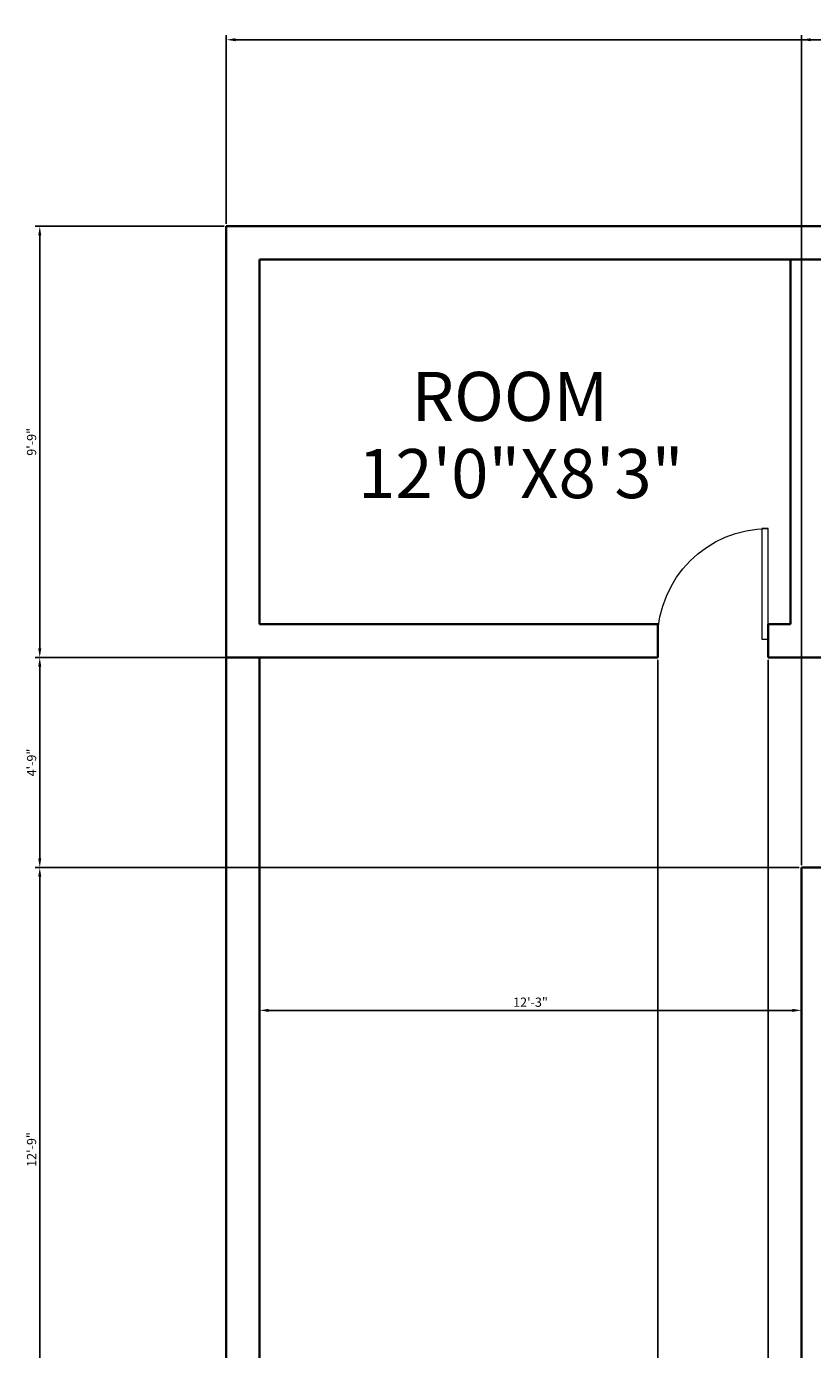
# Model space of a CAD drawing. Units: inches. Extents: x 3412 to 4225, y 13529 to 14581.
# Tile 4 of 7: x 3414 to 3627, y 14222 to 14581. Entities that reach past the tile are written whole.
import ezdxf

# ---------------------------------------------------------------- set-up
doc = ezdxf.new("R2010")
doc.units = ezdxf.units.IN
for name, color, linetype, lineweight in [('A-ANNO-DIMS', 2, 'Continuous', 13), ('A-AREA-IDEN', 7, 'Continuous', 18), ('A-DOOR', 4, 'Continuous', 18), ('A-WALL', 7, 'Continuous', 35), ('C-SITE-WALL', 7, 'Continuous', 35)]:
    doc.layers.add(name, color=color, linetype=linetype, lineweight=lineweight)
doc.styles.get("Standard").update_dxf_attribs({"font": 'arial.ttf'})
doc.dimstyles.new('ISO-25', dxfattribs={"dimtxt": 2.5, "dimasz": 2.5, "dimexe": 1.25, "dimexo": 0.625, "dimtad": 1, "dimdec": 0, "dimlunit": 3, "dimtxsty": 'Standard', "dimcen": 2.5, "dimadec": 0, "dimazin": 0, "dimtfac": 1, "dimtdec": 0, "dimtmove": 0, "dimatfit": 3, "dimfxl": 1, "dimarcsym": 0})

# ---------------------------------------------------------------- blocks, each defined once
blk = doc.blocks.new('*U3')
for p, q in [((0, 0), (0, -5)), ((30, 0), (30, -5))]:
    blk.add_line(p, q)
blk.add_lwpolyline([(0, 0), (0, 30), (1.75, 30), (1.75, 0)], close=True)
blk.add_arc((0, 0), 30, 0, 90)
blk = doc.blocks.new('*D21')
at = {"layer": 'A-ANNO-DIMS', "color": 0, "lineweight": -2, "transparency": 16777216}
for p, q in [((3477.36, 14351.81), (3477.36, 14312.43)), ((3624.36, 14351.81), (3624.36, 14312.43)), ((3621.86, 14313.68), (3479.86, 14313.68))]:
    blk.add_line(p, q, dxfattribs=at)
at = {"layer": 'A-ANNO-DIMS', "color": 0, "transparency": 16777216}
for points in [[(3479.86, 14314.1), (3479.86, 14313.26), (3477.36, 14313.68)], [(3621.86, 14314.1), (3621.86, 14313.26), (3624.36, 14313.68)]]:
    blk.add_solid(points, dxfattribs=at)
at = {"layer": 'Defpoints', "color": 0, "transparency": 16777216}
for p in [(3477.36, 14352.43), (3624.36, 14352.43), (3477.36, 14313.68)]:
    blk.add_point(p, dxfattribs=at)
at = {"layer": 'A-ANNO-DIMS', "color": 0, "transparency": 16777216, "insert": (3550.86, 14315.58), "char_height": 2.5, "attachment_point": 5}
blk.add_mtext('12\'-3"', dxfattribs=at)
blk = doc.blocks.new('*D56')
at = {"layer": 'A-ANNO-DIMS', "color": 0, "lineweight": -2, "transparency": 16777216}
for p, q in [((3468.36, 14527.06), (3468.36, 14578.28)), ((4173.36, 14527.06), (4173.36, 14578.28)), ((3470.86, 14577.03), (4170.86, 14577.03))]:
    blk.add_line(p, q, dxfattribs=at)
at = {"layer": 'A-ANNO-DIMS', "color": 0, "transparency": 16777216}
for points in [[(3470.86, 14577.45), (3470.86, 14576.62), (3468.36, 14577.03)], [(4170.86, 14577.45), (4170.86, 14576.62), (4173.36, 14577.03)]]:
    blk.add_solid(points, dxfattribs=at)
at = {"layer": 'Defpoints', "color": 0, "transparency": 16777216}
for p in [(4173.36, 14577.03), (3468.36, 14526.43), (4173.36, 14526.43)]:
    blk.add_point(p, dxfattribs=at)
at = {"layer": 'A-ANNO-DIMS', "color": 0, "transparency": 16777216, "insert": (3820.86, 14578.93), "char_height": 2.5, "attachment_point": 5}
blk.add_mtext('58\'-9"', dxfattribs=at)
blk = doc.blocks.new('*D58')
at = {"layer": 'A-ANNO-DIMS', "color": 0, "lineweight": -2, "transparency": 16777216}
for p, q in [((3467.73, 14526.43), (3416.51, 14526.43)), ((3417.76, 14523.93), (3417.76, 14411.93)), ((3467.73, 14409.43), (3416.51, 14409.43))]:
    blk.add_line(p, q, dxfattribs=at)
at = {"layer": 'A-ANNO-DIMS', "color": 0, "transparency": 16777216}
for points in [[(3417.34, 14523.93), (3418.17, 14523.93), (3417.76, 14526.43)], [(3417.34, 14411.93), (3418.17, 14411.93), (3417.76, 14409.43)]]:
    blk.add_solid(points, dxfattribs=at)
at = {"layer": 'Defpoints', "color": 0, "transparency": 16777216}
for p in [(3468.36, 14526.43), (3417.76, 14409.43), (3468.36, 14409.43)]:
    blk.add_point(p, dxfattribs=at)
at = {"layer": 'A-ANNO-DIMS', "color": 0, "transparency": 16777216, "insert": (3415.86, 14467.93), "char_height": 2.5, "attachment_point": 5, "rotation": 90}
blk.add_mtext('9\'-9"', dxfattribs=at)
blk = doc.blocks.new('*D59')
at = {"layer": 'A-ANNO-DIMS', "color": 0, "lineweight": -2, "transparency": 16777216}
for p, q in [((3468.36, 14527.06), (3468.36, 14578.28)), ((3936.36, 14518.06), (3936.36, 14578.28)), ((3470.86, 14577.03), (3933.86, 14577.03))]:
    blk.add_line(p, q, dxfattribs=at)
at = {"layer": 'A-ANNO-DIMS', "color": 0, "transparency": 16777216}
for points in [[(3470.86, 14577.45), (3470.86, 14576.62), (3468.36, 14577.03)], [(3933.86, 14577.45), (3933.86, 14576.62), (3936.36, 14577.03)]]:
    blk.add_solid(points, dxfattribs=at)
at = {"layer": 'Defpoints', "color": 0, "transparency": 16777216}
for p in [(3936.36, 14577.03), (3468.36, 14526.43), (3936.36, 14517.43)]:
    blk.add_point(p, dxfattribs=at)
at = {"layer": 'A-ANNO-DIMS', "color": 0, "transparency": 16777216, "insert": (3702.36, 14578.93), "char_height": 2.5, "attachment_point": 5}
blk.add_mtext('39\'-0"', dxfattribs=at)
blk = doc.blocks.new('*D60')
at = {"layer": 'A-ANNO-DIMS', "color": 0, "lineweight": -2, "transparency": 16777216}
for p, q in [((3584.73, 14409.43), (3416.51, 14409.43)), ((3417.76, 14354.93), (3417.76, 14406.93)), ((3623.73, 14352.43), (3416.51, 14352.43))]:
    blk.add_line(p, q, dxfattribs=at)
at = {"layer": 'A-ANNO-DIMS', "color": 0, "transparency": 16777216}
for points in [[(3417.34, 14406.93), (3418.17, 14406.93), (3417.76, 14409.43)], [(3417.34, 14354.93), (3418.17, 14354.93), (3417.76, 14352.43)]]:
    blk.add_solid(points, dxfattribs=at)
at = {"layer": 'Defpoints', "color": 0, "transparency": 16777216}
for p in [(3417.76, 14409.43), (3585.36, 14409.43), (3624.36, 14352.43)]:
    blk.add_point(p, dxfattribs=at)
at = {"layer": 'A-ANNO-DIMS', "color": 0, "transparency": 16777216, "insert": (3415.86, 14380.93), "char_height": 2.5, "attachment_point": 5, "rotation": 90}
blk.add_mtext('4\'-9"', dxfattribs=at)
blk = doc.blocks.new('*D61')
at = {"layer": 'A-ANNO-DIMS', "color": 0, "lineweight": -2, "transparency": 16777216}
for p, q in [((3477.36, 14408.81), (3477.36, 13550.58)), ((3585.36, 14408.81), (3585.36, 13550.58)), ((3479.86, 13551.83), (3582.86, 13551.83))]:
    blk.add_line(p, q, dxfattribs=at)
at = {"layer": 'A-ANNO-DIMS', "color": 0, "transparency": 16777216}
for points in [[(3479.86, 13552.25), (3479.86, 13551.42), (3477.36, 13551.83)], [(3582.86, 13552.25), (3582.86, 13551.42), (3585.36, 13551.83)]]:
    blk.add_solid(points, dxfattribs=at)
at = {"layer": 'Defpoints', "color": 0, "transparency": 16777216}
for p in [(3477.36, 14409.43), (3585.36, 14409.43), (3585.36, 13551.83)]:
    blk.add_point(p, dxfattribs=at)
at = {"layer": 'A-ANNO-DIMS', "color": 0, "transparency": 16777216, "insert": (3531.36, 13553.73), "char_height": 2.5, "attachment_point": 5}
blk.add_mtext('9\'-0"', dxfattribs=at)
blk = doc.blocks.new('*D62')
at = {"layer": 'A-ANNO-DIMS', "color": 0, "lineweight": -2, "transparency": 16777216}
for p, q in [((3585.36, 14408.81), (3585.36, 13550.58)), ((3615.36, 14408.81), (3615.36, 13550.58)), ((3587.86, 13551.83), (3612.86, 13551.83))]:
    blk.add_line(p, q, dxfattribs=at)
at = {"layer": 'A-ANNO-DIMS', "color": 0, "transparency": 16777216}
for points in [[(3587.86, 13552.25), (3587.86, 13551.42), (3585.36, 13551.83)], [(3612.86, 13552.25), (3612.86, 13551.42), (3615.36, 13551.83)]]:
    blk.add_solid(points, dxfattribs=at)
at = {"layer": 'Defpoints', "color": 0, "transparency": 16777216}
for p in [(3585.36, 14409.43), (3615.36, 14409.43), (3615.36, 13551.83)]:
    blk.add_point(p, dxfattribs=at)
at = {"layer": 'A-ANNO-DIMS', "color": 0, "transparency": 16777216, "insert": (3600.36, 13553.73), "char_height": 2.5, "attachment_point": 5}
blk.add_mtext('2\'-6"', dxfattribs=at)
blk = doc.blocks.new('*D63')
at = {"layer": 'A-ANNO-DIMS', "color": 0, "lineweight": -2, "transparency": 16777216}
for p, q in [((3615.36, 14408.81), (3615.36, 13550.58)), ((3738.36, 14408.81), (3738.36, 13550.58)), ((3617.86, 13551.83), (3735.86, 13551.83))]:
    blk.add_line(p, q, dxfattribs=at)
at = {"layer": 'A-ANNO-DIMS', "color": 0, "transparency": 16777216}
for points in [[(3617.86, 13552.25), (3617.86, 13551.42), (3615.36, 13551.83)], [(3735.86, 13552.25), (3735.86, 13551.42), (3738.36, 13551.83)]]:
    blk.add_solid(points, dxfattribs=at)
at = {"layer": 'Defpoints', "color": 0, "transparency": 16777216}
for p in [(3615.36, 14409.43), (3738.36, 14409.43), (3738.36, 13551.83)]:
    blk.add_point(p, dxfattribs=at)
at = {"layer": 'A-ANNO-DIMS', "color": 0, "transparency": 16777216, "insert": (3676.86, 13553.73), "char_height": 2.5, "attachment_point": 5}
blk.add_mtext('10\'-3"', dxfattribs=at)
blk = doc.blocks.new('*D68')
at = {"layer": 'A-ANNO-DIMS', "color": 0, "lineweight": -2, "transparency": 16777216}
for p, q in [((3624.36, 14353.06), (3624.36, 14578.28)), ((3679.38, 14353.06), (3679.38, 14578.28)), ((3626.86, 14577.03), (3676.88, 14577.03))]:
    blk.add_line(p, q, dxfattribs=at)
at = {"layer": 'A-ANNO-DIMS', "color": 0, "transparency": 16777216}
for points in [[(3626.86, 14577.45), (3626.86, 14576.62), (3624.36, 14577.03)], [(3676.88, 14577.45), (3676.88, 14576.62), (3679.38, 14577.03)]]:
    blk.add_solid(points, dxfattribs=at)
at = {"layer": 'Defpoints', "color": 0, "transparency": 16777216}
for p in [(3679.38, 14577.03), (3624.36, 14352.43), (3679.38, 14352.43)]:
    blk.add_point(p, dxfattribs=at)
at = {"layer": 'A-ANNO-DIMS', "color": 0, "transparency": 16777216, "insert": (3651.87, 14578.91), "char_height": 2.5, "attachment_point": 5}
blk.add_mtext('4\'-7"', dxfattribs=at)
blk = doc.blocks.new('*D73')
at = {"layer": 'A-ANNO-DIMS', "color": 0, "lineweight": -2, "transparency": 16777216}
for p, q in [((3623.73, 14352.43), (3416.51, 14352.43)), ((3417.76, 14349.93), (3417.76, 14201.93)), ((3593.73, 14199.43), (3416.51, 14199.43))]:
    blk.add_line(p, q, dxfattribs=at)
at = {"layer": 'A-ANNO-DIMS', "color": 0, "transparency": 16777216}
for points in [[(3417.34, 14349.93), (3418.17, 14349.93), (3417.76, 14352.43)], [(3417.34, 14201.93), (3418.17, 14201.93), (3417.76, 14199.43)]]:
    blk.add_solid(points, dxfattribs=at)
at = {"layer": 'Defpoints', "color": 0, "transparency": 16777216}
for p in [(3624.36, 14352.43), (3417.76, 14199.43), (3594.36, 14199.43)]:
    blk.add_point(p, dxfattribs=at)
at = {"layer": 'A-ANNO-DIMS', "color": 0, "transparency": 16777216, "insert": (3415.86, 14275.93), "char_height": 2.5, "attachment_point": 5, "rotation": 90}
blk.add_mtext('12\'-9"', dxfattribs=at)

msp = doc.modelspace()

# ---------------------------------------------------------------- linework, layer by layer
at = {"layer": 'A-WALL'}
for p, q in [((3477.36, 14517.43), (3477.36, 14418.43)), ((3621.36, 14517.43), (3621.36, 14418.43)), ((3477.36, 14418.43), (3585.36, 14418.43)), ((3585.36, 14418.43), (3585.36, 14409.43)), ((3615.36, 14418.43), (3615.36, 14409.43)), ((3615.36, 14418.43), (3621.36, 14418.43)), ((3468.36, 14409.43), (3585.36, 14409.43)), ((3615.36, 14409.43), (3738.36, 14409.43)), ((3624.36, 14352.43), (3624.36, 14199.43)), ((3624.36, 14352.43), (4092.36, 14352.43))]:
    msp.add_line(p, q, dxfattribs=at)
at = {"layer": 'C-SITE-WALL'}
for p, q in [((3468.36, 14526.43), (4173.36, 14526.43)), ((3468.36, 14526.43), (3468.36, 13602.43)), ((3477.36, 14517.43), (4164.36, 14517.43)), ((3477.36, 14409.43), (3477.36, 13611.43))]:
    msp.add_line(p, q, dxfattribs=at)

# ---------------------------------------------------------------- block references
at = {"layer": 'A-DOOR', "xscale": -1}
msp.add_blockref('*U3', (3615.36, 14414.43), dxfattribs=at)

# ---------------------------------------------------------------- texts
at = {"layer": 'A-AREA-IDEN'}
for s, p in [('ROOM', (3518.61, 14473.59)), ('12\'0"X8\'3"', (3504.11, 14452.66))]:
    msp.add_text(s, height=13.329, dxfattribs=at).set_placement(p)

# ---------------------------------------------------------------- dimensions: what is measured, and where the dimension line sits
at = {"layer": 'A-ANNO-DIMS'}
for base, p1, p2, override, picture, middle in [((4173.36, 14577.03), (3468.36, 14526.43), (4173.36, 14526.43), {"dimdec": 1, "dimlfac": 1, "dimrnd": 0, "dimzin": 1, "dimdsep": 46, "dimlunit": 4, "dimfrac": 2}, '*D56', (3820.86, 14578.93)), ((3936.36, 14577.03), (3468.36, 14526.43), (3936.36, 14517.43), {"dimdec": 1, "dimlfac": 1, "dimrnd": 0, "dimzin": 1, "dimdsep": 46, "dimlunit": 4, "dimfrac": 2}, '*D59', (3702.36, 14578.93)), ((3679.38, 14577.03), (3624.36, 14352.43), (3679.38, 14352.43), {"dimdec": 1, "dimlfac": 1, "dimrnd": 0, "dimzin": 1, "dimdsep": 46, "dimlunit": 4, "dimfrac": 2}, '*D68', (3651.87, 14578.91)), ((3585.36, 13551.83), (3477.36, 14409.43), (3585.36, 14409.43), {"dimdec": 1, "dimlfac": 1, "dimrnd": 0, "dimzin": 1, "dimdsep": 46, "dimlunit": 4, "dimfrac": 2}, '*D61', (3531.36, 13553.73)), ((3615.36, 13551.83), (3585.36, 14409.43), (3615.36, 14409.43), {"dimdec": 1, "dimlfac": 1, "dimrnd": 0, "dimzin": 1, "dimdsep": 46, "dimlunit": 4, "dimfrac": 2}, '*D62', (3600.36, 13553.73)), ((3738.36, 13551.83), (3615.36, 14409.43), (3738.36, 14409.43), {"dimdec": 1, "dimlfac": 1, "dimrnd": 0, "dimzin": 1, "dimdsep": 46, "dimlunit": 4, "dimfrac": 2}, '*D63', (3676.86, 13553.73)), ((3477.36, 14313.68), (3624.36, 14352.43), (3477.36, 14352.43), {"dimclrd": 0, "dimclre": 0, "dimclrt": 0}, '*D21', (3550.86, 14315.58))]:
    dim = msp.add_linear_dim(base=base, p1=p1, p2=p2, dimstyle='ISO-25', override=override, dxfattribs=at)
    dim.commit()
    dim.dimension.update_dxf_attribs({"geometry": picture, "text_midpoint": middle})
for base, p1, p2, picture, middle in [((3417.76, 14409.43), (3468.36, 14526.43), (3468.36, 14409.43), '*D58', (3415.86, 14467.93)), ((3417.76, 14409.43), (3624.36, 14352.43), (3585.36, 14409.43), '*D60', (3415.86, 14380.93)), ((3417.76, 14199.43), (3624.36, 14352.43), (3594.36, 14199.43), '*D73', (3415.86, 14275.93))]:
    dim = msp.add_linear_dim(base=base, p1=p1, p2=p2, angle=90, dimstyle='ISO-25', override={"dimdec": 1, "dimlfac": 1, "dimrnd": 0, "dimzin": 1, "dimdsep": 46, "dimlunit": 4, "dimfrac": 2}, dxfattribs=at)
    dim.commit()
    dim.dimension.update_dxf_attribs({"geometry": picture, "text_midpoint": middle})

doc.saveas('drawing.dxf')
